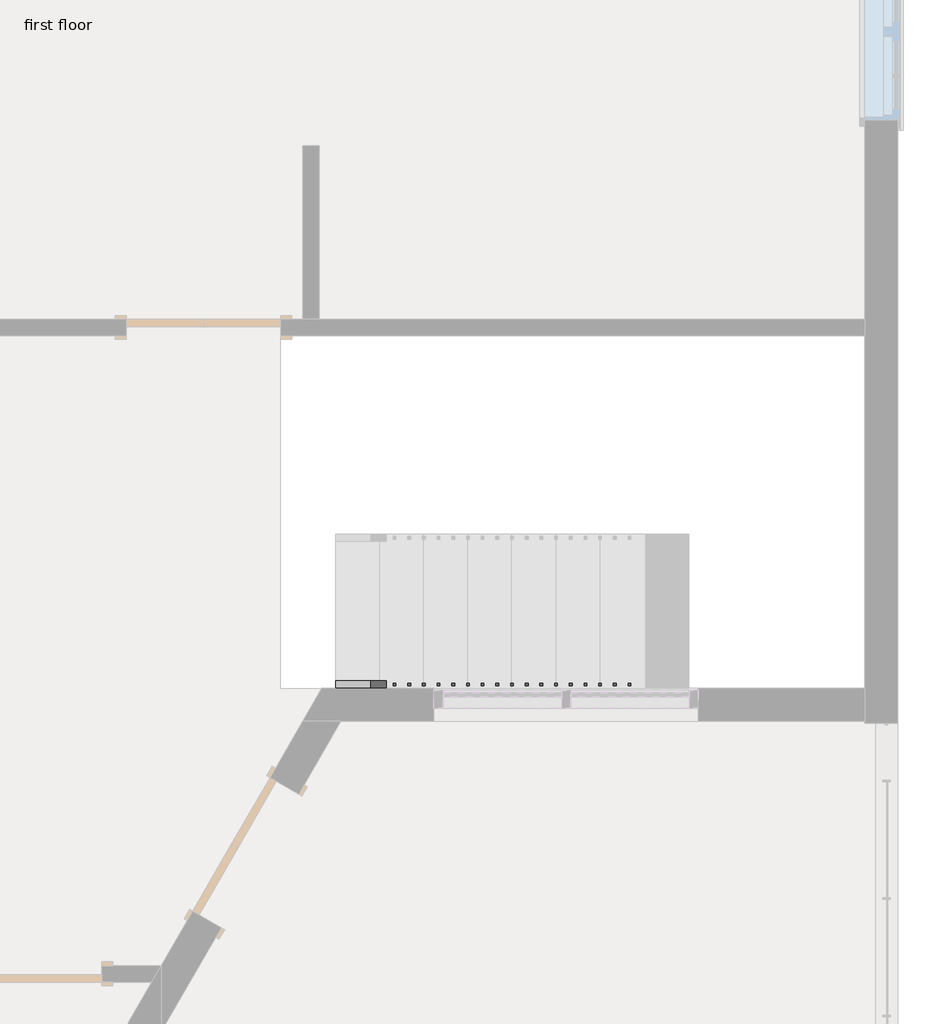
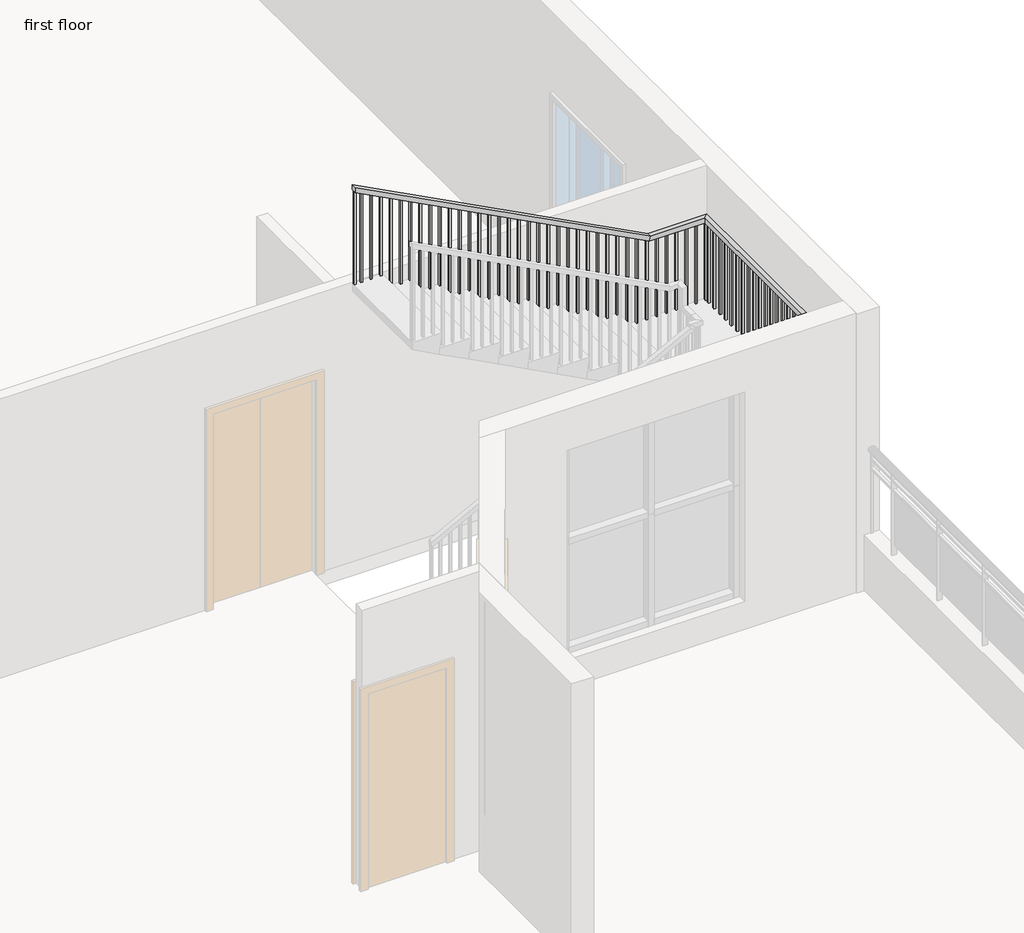
# One storey, part 3 of 4: 1 railing.
"""IFC4 building model written with IfcOpenShell, lengths in millimetres."""

from ifc_helpers import new_model, si_unit, frame, origin, place, context, project, spatial, polyline, outline, extrude, faceted_brep, element, save

model = new_model("IFC4")

# Units and contexts
model_context = context("Model", 3, world=origin())
ifc_project = project(units=[si_unit("LENGTHUNIT", "METRE", prefix="MILLI")], contexts=[model_context])

# Site, building, storey
site = spatial("IfcSite", under=ifc_project)
building = spatial("IfcBuilding", under=site)
storey = spatial("IfcBuildingStorey", under=building, Name="first floor", Elevation=3200.4)

# Railing
placement = place(None, origin())
element("IfcRailing", 1, ObjectType="Handrail - Rectangular", at=placement, inside=storey, context=model_context, shape_type="SolidModel", body=[
    faceted_brep([(1011.2585096, -3532.7523906, 4274.82), (1011.2585096, -3532.7523906, 4217.4446664), (1011.2585096, -3583.5523906, 4217.4446664), (1011.2585096, -3583.5523906, 4274.82), (3754.4585096, -3532.7523906, 5715.0), (3766.9829544, -3532.7523906, 5664.2), (3766.9829544, -3583.5523906, 5664.2), (3754.4585096, -3583.5523906, 5715.0), (4618.0585096, -3532.7523906, 5715.0), (4618.0585096, -3532.7523906, 5664.2), (4668.8585096, -3583.5523906, 5664.2), (4668.8585096, -3583.5523906, 5715.0), (4618.0585096, -1195.9523906, 5715.0), (4618.0585096, -1195.9523906, 5664.2), (4668.8585096, -1145.1523906, 5664.2), (4668.8585096, -1145.1523906, 5715.0), (4059.2585096, -1195.9523906, 5715.0), (4046.7340647, -1195.9523906, 5664.2), (4046.7340647, -1145.1523906, 5664.2), (4059.2585096, -1145.1523906, 5715.0), (1011.2585096, -1195.9523906, 7315.2), (1011.2585096, -1145.1523906, 7315.2), (1011.2585096, -1145.1523906, 7257.8246664), (1011.2585096, -1195.9523906, 7257.8246664)], [[[0, 1, 2, 3]], [[1, 0, 4, 5]], [[2, 1, 5, 6]], [[3, 2, 6, 7]], [[0, 3, 7, 4]], [[5, 4, 8, 9]], [[6, 5, 9, 10]], [[7, 6, 10, 11]], [[4, 7, 11, 8]], [[9, 8, 12, 13]], [[10, 9, 13, 14]], [[11, 10, 14, 15]], [[8, 11, 15, 12]], [[13, 12, 16, 17]], [[14, 13, 17, 18]], [[15, 14, 18, 19]], [[12, 15, 19, 16]], [[20, 21, 22, 23]], [[17, 16, 20, 23]], [[18, 17, 23, 22]], [[19, 18, 22, 21]], [[16, 19, 21, 20]]]),
    extrude(outline(polyline([(7212.8190414, 1096.9835096), (7222.8202914, 1077.9335096), (6240.78, 1077.9335096), (6240.78, 1096.9835096), (7212.8190414, 1096.9835096)])), frame((0.0, -1180.0773906, 0.0), z_axis=(0.0, 1.0, 0.0), x_axis=(0.0, 0.0, 1.0)), (0.0, 0.0, 1.0), 19.05),
    extrude(outline(polyline([(7159.4790414, 1198.5835096), (7169.4802914, 1179.5335096), (6240.78, 1179.5335096), (6240.78, 1198.5835096), (7159.4790414, 1198.5835096)])), frame((0.0, -1180.0773906, 0.0), z_axis=(0.0, 1.0, 0.0), x_axis=(0.0, 0.0, 1.0)), (0.0, 0.0, 1.0), 19.05),
    extrude(outline(polyline([(7106.1390414, 1300.1835096), (7116.1402914, 1281.1335096), (6240.78, 1281.1335096), (6240.78, 1300.1835096), (7106.1390414, 1300.1835096)])), frame((0.0, -1180.0773906, 0.0), z_axis=(0.0, 1.0, 0.0), x_axis=(0.0, 0.0, 1.0)), (0.0, 0.0, 1.0), 19.05),
    extrude(outline(polyline([(7052.7990414, 1401.7835096), (7062.8002914, 1382.7335096), (6080.76, 1382.7335096), (6080.76, 1401.7835096), (7052.7990414, 1401.7835096)])), frame((0.0, -1180.0773906, 0.0), z_axis=(0.0, 1.0, 0.0), x_axis=(0.0, 0.0, 1.0)), (0.0, 0.0, 1.0), 19.05),
    extrude(outline(polyline([(6999.4590414, 1503.3835096), (7009.4602914, 1484.3335096), (6080.76, 1484.3335096), (6080.76, 1503.3835096), (6999.4590414, 1503.3835096)])), frame((0.0, -1180.0773906, 0.0), z_axis=(0.0, 1.0, 0.0), x_axis=(0.0, 0.0, 1.0)), (0.0, 0.0, 1.0), 19.05),
    extrude(outline(polyline([(6946.1190414, 1604.9835096), (6956.1202914, 1585.9335096), (6080.76, 1585.9335096), (6080.76, 1604.9835096), (6946.1190414, 1604.9835096)])), frame((0.0, -1180.0773906, 0.0), z_axis=(0.0, 1.0, 0.0), x_axis=(0.0, 0.0, 1.0)), (0.0, 0.0, 1.0), 19.05),
    extrude(outline(polyline([(6892.7790414, 1706.5835096), (6902.7802914, 1687.5335096), (5920.74, 1687.5335096), (5920.74, 1706.5835096), (6892.7790414, 1706.5835096)])), frame((0.0, -1180.0773906, 0.0), z_axis=(0.0, 1.0, 0.0), x_axis=(0.0, 0.0, 1.0)), (0.0, 0.0, 1.0), 19.05),
    extrude(outline(polyline([(6839.4390414, 1808.1835096), (6849.4402914, 1789.1335096), (5920.74, 1789.1335096), (5920.74, 1808.1835096), (6839.4390414, 1808.1835096)])), frame((0.0, -1180.0773906, 0.0), z_axis=(0.0, 1.0, 0.0), x_axis=(0.0, 0.0, 1.0)), (0.0, 0.0, 1.0), 19.05),
    extrude(outline(polyline([(6786.0990414, 1909.7835096), (6796.1002914, 1890.7335096), (5920.74, 1890.7335096), (5920.74, 1909.7835096), (6786.0990414, 1909.7835096)])), frame((0.0, -1180.0773906, 0.0), z_axis=(0.0, 1.0, 0.0), x_axis=(0.0, 0.0, 1.0)), (0.0, 0.0, 1.0), 19.05),
    extrude(outline(polyline([(6732.7590414, 2011.3835096), (6742.7602914, 1992.3335096), (5760.72, 1992.3335096), (5760.72, 2011.3835096), (6732.7590414, 2011.3835096)])), frame((0.0, -1180.0773906, 0.0), z_axis=(0.0, 1.0, 0.0), x_axis=(0.0, 0.0, 1.0)), (0.0, 0.0, 1.0), 19.05),
    extrude(outline(polyline([(6679.4190414, 2112.9835096), (6689.4202914, 2093.9335096), (5760.72, 2093.9335096), (5760.72, 2112.9835096), (6679.4190414, 2112.9835096)])), frame((0.0, -1180.0773906, 0.0), z_axis=(0.0, 1.0, 0.0), x_axis=(0.0, 0.0, 1.0)), (0.0, 0.0, 1.0), 19.05),
    extrude(outline(polyline([(6626.0790414, 2214.5835096), (6636.0802914, 2195.5335096), (5760.72, 2195.5335096), (5760.72, 2214.5835096), (6626.0790414, 2214.5835096)])), frame((0.0, -1180.0773906, 0.0), z_axis=(0.0, 1.0, 0.0), x_axis=(0.0, 0.0, 1.0)), (0.0, 0.0, 1.0), 19.05),
    extrude(outline(polyline([(6572.7390414, 2316.1835096), (6582.7402914, 2297.1335096), (5600.7, 2297.1335096), (5600.7, 2316.1835096), (6572.7390414, 2316.1835096)])), frame((0.0, -1180.0773906, 0.0), z_axis=(0.0, 1.0, 0.0), x_axis=(0.0, 0.0, 1.0)), (0.0, 0.0, 1.0), 19.05),
    extrude(outline(polyline([(6519.3990414, 2417.7835096), (6529.4002914, 2398.7335096), (5600.7, 2398.7335096), (5600.7, 2417.7835096), (6519.3990414, 2417.7835096)])), frame((0.0, -1180.0773906, 0.0), z_axis=(0.0, 1.0, 0.0), x_axis=(0.0, 0.0, 1.0)), (0.0, 0.0, 1.0), 19.05),
    extrude(outline(polyline([(6466.0590414, 2519.3835096), (6476.0602914, 2500.3335096), (5600.7, 2500.3335096), (5600.7, 2519.3835096), (6466.0590414, 2519.3835096)])), frame((0.0, -1180.0773906, 0.0), z_axis=(0.0, 1.0, 0.0), x_axis=(0.0, 0.0, 1.0)), (0.0, 0.0, 1.0), 19.05),
    extrude(outline(polyline([(6412.7190414, 2620.9835096), (6422.7202914, 2601.9335096), (5440.68, 2601.9335096), (5440.68, 2620.9835096), (6412.7190414, 2620.9835096)])), frame((0.0, -1180.0773906, 0.0), z_axis=(0.0, 1.0, 0.0), x_axis=(0.0, 0.0, 1.0)), (0.0, 0.0, 1.0), 19.05),
    extrude(outline(polyline([(6359.3790414, 2722.5835096), (6369.3802914, 2703.5335096), (5440.68, 2703.5335096), (5440.68, 2722.5835096), (6359.3790414, 2722.5835096)])), frame((0.0, -1180.0773906, 0.0), z_axis=(0.0, 1.0, 0.0), x_axis=(0.0, 0.0, 1.0)), (0.0, 0.0, 1.0), 19.05),
    extrude(outline(polyline([(6306.0390414, 2824.1835096), (6316.0402914, 2805.1335096), (5440.68, 2805.1335096), (5440.68, 2824.1835096), (6306.0390414, 2824.1835096)])), frame((0.0, -1180.0773906, 0.0), z_axis=(0.0, 1.0, 0.0), x_axis=(0.0, 0.0, 1.0)), (0.0, 0.0, 1.0), 19.05),
    extrude(outline(polyline([(6252.6990414, 2925.7835096), (6262.7002914, 2906.7335096), (5280.66, 2906.7335096), (5280.66, 2925.7835096), (6252.6990414, 2925.7835096)])), frame((0.0, -1180.0773906, 0.0), z_axis=(0.0, 1.0, 0.0), x_axis=(0.0, 0.0, 1.0)), (0.0, 0.0, 1.0), 19.05),
    extrude(outline(polyline([(6199.3590414, 3027.3835096), (6209.3602914, 3008.3335096), (5280.66, 3008.3335096), (5280.66, 3027.3835096), (6199.3590414, 3027.3835096)])), frame((0.0, -1180.0773906, 0.0), z_axis=(0.0, 1.0, 0.0), x_axis=(0.0, 0.0, 1.0)), (0.0, 0.0, 1.0), 19.05),
    extrude(outline(polyline([(6146.0190414, 3128.9835096), (6156.0202914, 3109.9335096), (5280.66, 3109.9335096), (5280.66, 3128.9835096), (6146.0190414, 3128.9835096)])), frame((0.0, -1180.0773906, 0.0), z_axis=(0.0, 1.0, 0.0), x_axis=(0.0, 0.0, 1.0)), (0.0, 0.0, 1.0), 19.05),
    extrude(outline(polyline([(6092.6790414, 3230.5835096), (6102.6802914, 3211.5335096), (5120.64, 3211.5335096), (5120.64, 3230.5835096), (6092.6790414, 3230.5835096)])), frame((0.0, -1180.0773906, 0.0), z_axis=(0.0, 1.0, 0.0), x_axis=(0.0, 0.0, 1.0)), (0.0, 0.0, 1.0), 19.05),
    extrude(outline(polyline([(6039.3390414, 3332.1835096), (6049.3402914, 3313.1335096), (5120.64, 3313.1335096), (5120.64, 3332.1835096), (6039.3390414, 3332.1835096)])), frame((0.0, -1180.0773906, 0.0), z_axis=(0.0, 1.0, 0.0), x_axis=(0.0, 0.0, 1.0)), (0.0, 0.0, 1.0), 19.05),
    extrude(outline(polyline([(5985.9990414, 3433.7835096), (5996.0002914, 3414.7335096), (5120.64, 3414.7335096), (5120.64, 3433.7835096), (5985.9990414, 3433.7835096)])), frame((0.0, -1180.0773906, 0.0), z_axis=(0.0, 1.0, 0.0), x_axis=(0.0, 0.0, 1.0)), (0.0, 0.0, 1.0), 19.05),
    extrude(outline(polyline([(5932.6590414, 3535.3835096), (5942.6602914, 3516.3335096), (4960.62, 3516.3335096), (4960.62, 3535.3835096), (5932.6590414, 3535.3835096)])), frame((0.0, -1180.0773906, 0.0), z_axis=(0.0, 1.0, 0.0), x_axis=(0.0, 0.0, 1.0)), (0.0, 0.0, 1.0), 19.05),
    extrude(outline(polyline([(5879.3190414, 3636.9835096), (5889.3202914, 3617.9335096), (4960.62, 3617.9335096), (4960.62, 3636.9835096), (5879.3190414, 3636.9835096)])), frame((0.0, -1180.0773906, 0.0), z_axis=(0.0, 1.0, 0.0), x_axis=(0.0, 0.0, 1.0)), (0.0, 0.0, 1.0), 19.05),
    extrude(outline(polyline([(5825.9790414, 3738.5835096), (5835.9802914, 3719.5335096), (4960.62, 3719.5335096), (4960.62, 3738.5835096), (5825.9790414, 3738.5835096)])), frame((0.0, -1180.0773906, 0.0), z_axis=(0.0, 1.0, 0.0), x_axis=(0.0, 0.0, 1.0)), (0.0, 0.0, 1.0), 19.05),
    extrude(outline(polyline([(5772.6390414, 3840.1835096), (5782.6402914, 3821.1335096), (4800.6, 3821.1335096), (4800.6, 3840.1835096), (5772.6390414, 3840.1835096)])), frame((0.0, -1180.0773906, 0.0), z_axis=(0.0, 1.0, 0.0), x_axis=(0.0, 0.0, 1.0)), (0.0, 0.0, 1.0), 19.05),
    extrude(outline(polyline([(5719.2990414, 3941.7835096), (5729.3002914, 3922.7335096), (4800.6, 3922.7335096), (4800.6, 3941.7835096), (5719.2990414, 3941.7835096)])), frame((0.0, -1180.0773906, 0.0), z_axis=(0.0, 1.0, 0.0), x_axis=(0.0, 0.0, 1.0)), (0.0, 0.0, 1.0), 19.05),
    extrude(outline(polyline([(5665.9590414, 4043.3835096), (5675.9602914, 4024.3335096), (4800.6, 4024.3335096), (4800.6, 4043.3835096), (5665.9590414, 4043.3835096)])), frame((0.0, -1180.0773906, 0.0), z_axis=(0.0, 1.0, 0.0), x_axis=(0.0, 0.0, 1.0)), (0.0, 0.0, 1.0), 19.05),
    extrude(outline(polyline([(4144.9835096, -1161.0273906), (4144.9835096, -1180.0773906), (4125.9335096, -1180.0773906), (4125.9335096, -1161.0273906), (4144.9835096, -1161.0273906)])), frame((0.0, 0.0, 4800.6), z_axis=(0.0, 0.0, 1.0), x_axis=(1.0, 0.0, 0.0)), (0.0, 0.0, 1.0), 863.6),
    extrude(outline(polyline([(4246.5835096, -1161.0273906), (4246.5835096, -1180.0773906), (4227.5335096, -1180.0773906), (4227.5335096, -1161.0273906), (4246.5835096, -1161.0273906)])), frame((0.0, 0.0, 4800.6), z_axis=(0.0, 0.0, 1.0), x_axis=(1.0, 0.0, 0.0)), (0.0, 0.0, 1.0), 863.6),
    extrude(outline(polyline([(4348.1835096, -1161.0273906), (4348.1835096, -1180.0773906), (4329.1335096, -1180.0773906), (4329.1335096, -1161.0273906), (4348.1835096, -1161.0273906)])), frame((0.0, 0.0, 4800.6), z_axis=(0.0, 0.0, 1.0), x_axis=(1.0, 0.0, 0.0)), (0.0, 0.0, 1.0), 863.6),
    extrude(outline(polyline([(4449.7835096, -1161.0273906), (4449.7835096, -1180.0773906), (4430.7335096, -1180.0773906), (4430.7335096, -1161.0273906), (4449.7835096, -1161.0273906)])), frame((0.0, 0.0, 4800.6), z_axis=(0.0, 0.0, 1.0), x_axis=(1.0, 0.0, 0.0)), (0.0, 0.0, 1.0), 863.6),
    extrude(outline(polyline([(4551.3835096, -1161.0273906), (4551.3835096, -1180.0773906), (4532.3335096, -1180.0773906), (4532.3335096, -1161.0273906), (4551.3835096, -1161.0273906)])), frame((0.0, 0.0, 4800.6), z_axis=(0.0, 0.0, 1.0), x_axis=(1.0, 0.0, 0.0)), (0.0, 0.0, 1.0), 863.6),
    extrude(outline(polyline([(4652.9835096, -1230.8773906), (4633.9335096, -1230.8773906), (4633.9335096, -1211.8273906), (4652.9835096, -1211.8273906), (4652.9835096, -1230.8773906)])), frame((0.0, 0.0, 4800.6), z_axis=(0.0, 0.0, 1.0), x_axis=(1.0, 0.0, 0.0)), (0.0, 0.0, 1.0), 863.6),
    extrude(outline(polyline([(4652.9835096, -1332.4773906), (4633.9335096, -1332.4773906), (4633.9335096, -1313.4273906), (4652.9835096, -1313.4273906), (4652.9835096, -1332.4773906)])), frame((0.0, 0.0, 4800.6), z_axis=(0.0, 0.0, 1.0), x_axis=(1.0, 0.0, 0.0)), (0.0, 0.0, 1.0), 863.6),
    extrude(outline(polyline([(4652.9835096, -1434.0773906), (4633.9335096, -1434.0773906), (4633.9335096, -1415.0273906), (4652.9835096, -1415.0273906), (4652.9835096, -1434.0773906)])), frame((0.0, 0.0, 4800.6), z_axis=(0.0, 0.0, 1.0), x_axis=(1.0, 0.0, 0.0)), (0.0, 0.0, 1.0), 863.6),
    extrude(outline(polyline([(4652.9835096, -1535.6773906), (4633.9335096, -1535.6773906), (4633.9335096, -1516.6273906), (4652.9835096, -1516.6273906), (4652.9835096, -1535.6773906)])), frame((0.0, 0.0, 4800.6), z_axis=(0.0, 0.0, 1.0), x_axis=(1.0, 0.0, 0.0)), (0.0, 0.0, 1.0), 863.6),
    extrude(outline(polyline([(4652.9835096, -1637.2773906), (4633.9335096, -1637.2773906), (4633.9335096, -1618.2273906), (4652.9835096, -1618.2273906), (4652.9835096, -1637.2773906)])), frame((0.0, 0.0, 4800.6), z_axis=(0.0, 0.0, 1.0), x_axis=(1.0, 0.0, 0.0)), (0.0, 0.0, 1.0), 863.6),
    extrude(outline(polyline([(4652.9835096, -1738.8773906), (4633.9335096, -1738.8773906), (4633.9335096, -1719.8273906), (4652.9835096, -1719.8273906), (4652.9835096, -1738.8773906)])), frame((0.0, 0.0, 4800.6), z_axis=(0.0, 0.0, 1.0), x_axis=(1.0, 0.0, 0.0)), (0.0, 0.0, 1.0), 863.6),
    extrude(outline(polyline([(4652.9835096, -1840.4773906), (4633.9335096, -1840.4773906), (4633.9335096, -1821.4273906), (4652.9835096, -1821.4273906), (4652.9835096, -1840.4773906)])), frame((0.0, 0.0, 4800.6), z_axis=(0.0, 0.0, 1.0), x_axis=(1.0, 0.0, 0.0)), (0.0, 0.0, 1.0), 863.6),
    extrude(outline(polyline([(4652.9835096, -1942.0773906), (4633.9335096, -1942.0773906), (4633.9335096, -1923.0273906), (4652.9835096, -1923.0273906), (4652.9835096, -1942.0773906)])), frame((0.0, 0.0, 4800.6), z_axis=(0.0, 0.0, 1.0), x_axis=(1.0, 0.0, 0.0)), (0.0, 0.0, 1.0), 863.6),
    extrude(outline(polyline([(4652.9835096, -2043.6773906), (4633.9335096, -2043.6773906), (4633.9335096, -2024.6273906), (4652.9835096, -2024.6273906), (4652.9835096, -2043.6773906)])), frame((0.0, 0.0, 4800.6), z_axis=(0.0, 0.0, 1.0), x_axis=(1.0, 0.0, 0.0)), (0.0, 0.0, 1.0), 863.6),
    extrude(outline(polyline([(4652.9835096, -2145.2773906), (4633.9335096, -2145.2773906), (4633.9335096, -2126.2273906), (4652.9835096, -2126.2273906), (4652.9835096, -2145.2773906)])), frame((0.0, 0.0, 4800.6), z_axis=(0.0, 0.0, 1.0), x_axis=(1.0, 0.0, 0.0)), (0.0, 0.0, 1.0), 863.6),
    extrude(outline(polyline([(4652.9835096, -2246.8773906), (4633.9335096, -2246.8773906), (4633.9335096, -2227.8273906), (4652.9835096, -2227.8273906), (4652.9835096, -2246.8773906)])), frame((0.0, 0.0, 4800.6), z_axis=(0.0, 0.0, 1.0), x_axis=(1.0, 0.0, 0.0)), (0.0, 0.0, 1.0), 863.6),
    extrude(outline(polyline([(4652.9835096, -2348.4773906), (4633.9335096, -2348.4773906), (4633.9335096, -2329.4273906), (4652.9835096, -2329.4273906), (4652.9835096, -2348.4773906)])), frame((0.0, 0.0, 4800.6), z_axis=(0.0, 0.0, 1.0), x_axis=(1.0, 0.0, 0.0)), (0.0, 0.0, 1.0), 863.6),
    extrude(outline(polyline([(4652.9835096, -2450.0773906), (4633.9335096, -2450.0773906), (4633.9335096, -2431.0273906), (4652.9835096, -2431.0273906), (4652.9835096, -2450.0773906)])), frame((0.0, 0.0, 4800.6), z_axis=(0.0, 0.0, 1.0), x_axis=(1.0, 0.0, 0.0)), (0.0, 0.0, 1.0), 863.6),
    extrude(outline(polyline([(4652.9835096, -2551.6773906), (4633.9335096, -2551.6773906), (4633.9335096, -2532.6273906), (4652.9835096, -2532.6273906), (4652.9835096, -2551.6773906)])), frame((0.0, 0.0, 4800.6), z_axis=(0.0, 0.0, 1.0), x_axis=(1.0, 0.0, 0.0)), (0.0, 0.0, 1.0), 863.6),
    extrude(outline(polyline([(4652.9835096, -2653.2773906), (4633.9335096, -2653.2773906), (4633.9335096, -2634.2273906), (4652.9835096, -2634.2273906), (4652.9835096, -2653.2773906)])), frame((0.0, 0.0, 4800.6), z_axis=(0.0, 0.0, 1.0), x_axis=(1.0, 0.0, 0.0)), (0.0, 0.0, 1.0), 863.6),
    extrude(outline(polyline([(4652.9835096, -2754.8773906), (4633.9335096, -2754.8773906), (4633.9335096, -2735.8273906), (4652.9835096, -2735.8273906), (4652.9835096, -2754.8773906)])), frame((0.0, 0.0, 4800.6), z_axis=(0.0, 0.0, 1.0), x_axis=(1.0, 0.0, 0.0)), (0.0, 0.0, 1.0), 863.6),
    extrude(outline(polyline([(4652.9835096, -2856.4773906), (4633.9335096, -2856.4773906), (4633.9335096, -2837.4273906), (4652.9835096, -2837.4273906), (4652.9835096, -2856.4773906)])), frame((0.0, 0.0, 4800.6), z_axis=(0.0, 0.0, 1.0), x_axis=(1.0, 0.0, 0.0)), (0.0, 0.0, 1.0), 863.6),
    extrude(outline(polyline([(4652.9835096, -2958.0773906), (4633.9335096, -2958.0773906), (4633.9335096, -2939.0273906), (4652.9835096, -2939.0273906), (4652.9835096, -2958.0773906)])), frame((0.0, 0.0, 4800.6), z_axis=(0.0, 0.0, 1.0), x_axis=(1.0, 0.0, 0.0)), (0.0, 0.0, 1.0), 863.6),
    extrude(outline(polyline([(4652.9835096, -3059.6773906), (4633.9335096, -3059.6773906), (4633.9335096, -3040.6273906), (4652.9835096, -3040.6273906), (4652.9835096, -3059.6773906)])), frame((0.0, 0.0, 4800.6), z_axis=(0.0, 0.0, 1.0), x_axis=(1.0, 0.0, 0.0)), (0.0, 0.0, 1.0), 863.6),
    extrude(outline(polyline([(4652.9835096, -3161.2773906), (4633.9335096, -3161.2773906), (4633.9335096, -3142.2273906), (4652.9835096, -3142.2273906), (4652.9835096, -3161.2773906)])), frame((0.0, 0.0, 4800.6), z_axis=(0.0, 0.0, 1.0), x_axis=(1.0, 0.0, 0.0)), (0.0, 0.0, 1.0), 863.6),
    extrude(outline(polyline([(4652.9835096, -3262.8773906), (4633.9335096, -3262.8773906), (4633.9335096, -3243.8273906), (4652.9835096, -3243.8273906), (4652.9835096, -3262.8773906)])), frame((0.0, 0.0, 4800.6), z_axis=(0.0, 0.0, 1.0), x_axis=(1.0, 0.0, 0.0)), (0.0, 0.0, 1.0), 863.6),
    extrude(outline(polyline([(4652.9835096, -3364.4773906), (4633.9335096, -3364.4773906), (4633.9335096, -3345.4273906), (4652.9835096, -3345.4273906), (4652.9835096, -3364.4773906)])), frame((0.0, 0.0, 4800.6), z_axis=(0.0, 0.0, 1.0), x_axis=(1.0, 0.0, 0.0)), (0.0, 0.0, 1.0), 863.6),
    extrude(outline(polyline([(4652.9835096, -3466.0773906), (4633.9335096, -3466.0773906), (4633.9335096, -3447.0273906), (4652.9835096, -3447.0273906), (4652.9835096, -3466.0773906)])), frame((0.0, 0.0, 4800.6), z_axis=(0.0, 0.0, 1.0), x_axis=(1.0, 0.0, 0.0)), (0.0, 0.0, 1.0), 863.6),
    extrude(outline(polyline([(4557.7335096, -3567.6773906), (4557.7335096, -3548.6273906), (4576.7835096, -3548.6273906), (4576.7835096, -3567.6773906), (4557.7335096, -3567.6773906)])), frame((0.0, 0.0, 4800.6), z_axis=(0.0, 0.0, 1.0), x_axis=(1.0, 0.0, 0.0)), (0.0, 0.0, 1.0), 863.6),
    extrude(outline(polyline([(4456.1335096, -3567.6773906), (4456.1335096, -3548.6273906), (4475.1835096, -3548.6273906), (4475.1835096, -3567.6773906), (4456.1335096, -3567.6773906)])), frame((0.0, 0.0, 4800.6), z_axis=(0.0, 0.0, 1.0), x_axis=(1.0, 0.0, 0.0)), (0.0, 0.0, 1.0), 863.6),
    extrude(outline(polyline([(4354.5335096, -3567.6773906), (4354.5335096, -3548.6273906), (4373.5835096, -3548.6273906), (4373.5835096, -3567.6773906), (4354.5335096, -3567.6773906)])), frame((0.0, 0.0, 4800.6), z_axis=(0.0, 0.0, 1.0), x_axis=(1.0, 0.0, 0.0)), (0.0, 0.0, 1.0), 863.6),
    extrude(outline(polyline([(4252.9335096, -3567.6773906), (4252.9335096, -3548.6273906), (4271.9835096, -3548.6273906), (4271.9835096, -3567.6773906), (4252.9335096, -3567.6773906)])), frame((0.0, 0.0, 4800.6), z_axis=(0.0, 0.0, 1.0), x_axis=(1.0, 0.0, 0.0)), (0.0, 0.0, 1.0), 863.6),
    extrude(outline(polyline([(4151.3335096, -3567.6773906), (4151.3335096, -3548.6273906), (4170.3835096, -3548.6273906), (4170.3835096, -3567.6773906), (4151.3335096, -3567.6773906)])), frame((0.0, 0.0, 4800.6), z_axis=(0.0, 0.0, 1.0), x_axis=(1.0, 0.0, 0.0)), (0.0, 0.0, 1.0), 863.6),
    extrude(outline(polyline([(4049.7335096, -3567.6773906), (4049.7335096, -3548.6273906), (4068.7835096, -3548.6273906), (4068.7835096, -3567.6773906), (4049.7335096, -3567.6773906)])), frame((0.0, 0.0, 4800.6), z_axis=(0.0, 0.0, 1.0), x_axis=(1.0, 0.0, 0.0)), (0.0, 0.0, 1.0), 863.6),
    extrude(outline(polyline([(3948.1335096, -3567.6773906), (3948.1335096, -3548.6273906), (3967.1835096, -3548.6273906), (3967.1835096, -3567.6773906), (3948.1335096, -3567.6773906)])), frame((0.0, 0.0, 4800.6), z_axis=(0.0, 0.0, 1.0), x_axis=(1.0, 0.0, 0.0)), (0.0, 0.0, 1.0), 863.6),
    extrude(outline(polyline([(3846.5335096, -3567.6773906), (3846.5335096, -3548.6273906), (3865.5835096, -3548.6273906), (3865.5835096, -3567.6773906), (3846.5335096, -3567.6773906)])), frame((0.0, 0.0, 4800.6), z_axis=(0.0, 0.0, 1.0), x_axis=(1.0, 0.0, 0.0)), (0.0, 0.0, 1.0), 863.6),
    extrude(outline(polyline([(5662.6252914, 3763.9835096), (5652.6240414, 3744.9335096), (4800.6, 3744.9335096), (4800.6, 3763.9835096), (5662.6252914, 3763.9835096)])), frame((0.0, -3567.6773906, 0.0), z_axis=(0.0, 1.0, 0.0), x_axis=(0.0, 0.0, 1.0)), (0.0, 0.0, 1.0), 19.05),
    extrude(outline(polyline([(5609.2852914, 3662.3835096), (5599.2840414, 3643.3335096), (4640.58, 3643.3335096), (4640.58, 3662.3835096), (5609.2852914, 3662.3835096)])), frame((0.0, -3567.6773906, 0.0), z_axis=(0.0, 1.0, 0.0), x_axis=(0.0, 0.0, 1.0)), (0.0, 0.0, 1.0), 19.05),
    extrude(outline(polyline([(5555.9452914, 3560.7835096), (5545.9440414, 3541.7335096), (4640.58, 3541.7335096), (4640.58, 3560.7835096), (5555.9452914, 3560.7835096)])), frame((0.0, -3567.6773906, 0.0), z_axis=(0.0, 1.0, 0.0), x_axis=(0.0, 0.0, 1.0)), (0.0, 0.0, 1.0), 19.05),
    extrude(outline(polyline([(5502.6052914, 3459.1835096), (5492.6040414, 3440.1335096), (4640.58, 3440.1335096), (4640.58, 3459.1835096), (5502.6052914, 3459.1835096)])), frame((0.0, -3567.6773906, 0.0), z_axis=(0.0, 1.0, 0.0), x_axis=(0.0, 0.0, 1.0)), (0.0, 0.0, 1.0), 19.05),
    extrude(outline(polyline([(5449.2652914, 3357.5835096), (5439.2640414, 3338.5335096), (4480.56, 3338.5335096), (4480.56, 3357.5835096), (5449.2652914, 3357.5835096)])), frame((0.0, -3567.6773906, 0.0), z_axis=(0.0, 1.0, 0.0), x_axis=(0.0, 0.0, 1.0)), (0.0, 0.0, 1.0), 19.05),
    extrude(outline(polyline([(5395.9252914, 3255.9835096), (5385.9240414, 3236.9335096), (4480.56, 3236.9335096), (4480.56, 3255.9835096), (5395.9252914, 3255.9835096)])), frame((0.0, -3567.6773906, 0.0), z_axis=(0.0, 1.0, 0.0), x_axis=(0.0, 0.0, 1.0)), (0.0, 0.0, 1.0), 19.05),
    extrude(outline(polyline([(5342.5852914, 3154.3835096), (5332.5840414, 3135.3335096), (4480.56, 3135.3335096), (4480.56, 3154.3835096), (5342.5852914, 3154.3835096)])), frame((0.0, -3567.6773906, 0.0), z_axis=(0.0, 1.0, 0.0), x_axis=(0.0, 0.0, 1.0)), (0.0, 0.0, 1.0), 19.05),
    extrude(outline(polyline([(5289.2452914, 3052.7835096), (5279.2440414, 3033.7335096), (4320.54, 3033.7335096), (4320.54, 3052.7835096), (5289.2452914, 3052.7835096)])), frame((0.0, -3567.6773906, 0.0), z_axis=(0.0, 1.0, 0.0), x_axis=(0.0, 0.0, 1.0)), (0.0, 0.0, 1.0), 19.05),
    extrude(outline(polyline([(5235.9052914, 2951.1835096), (5225.9040414, 2932.1335096), (4320.54, 2932.1335096), (4320.54, 2951.1835096), (5235.9052914, 2951.1835096)])), frame((0.0, -3567.6773906, 0.0), z_axis=(0.0, 1.0, 0.0), x_axis=(0.0, 0.0, 1.0)), (0.0, 0.0, 1.0), 19.05),
    extrude(outline(polyline([(5182.5652914, 2849.5835096), (5172.5640414, 2830.5335096), (4320.54, 2830.5335096), (4320.54, 2849.5835096), (5182.5652914, 2849.5835096)])), frame((0.0, -3567.6773906, 0.0), z_axis=(0.0, 1.0, 0.0), x_axis=(0.0, 0.0, 1.0)), (0.0, 0.0, 1.0), 19.05),
    extrude(outline(polyline([(5129.2252914, 2747.9835096), (5119.2240414, 2728.9335096), (4160.52, 2728.9335096), (4160.52, 2747.9835096), (5129.2252914, 2747.9835096)])), frame((0.0, -3567.6773906, 0.0), z_axis=(0.0, 1.0, 0.0), x_axis=(0.0, 0.0, 1.0)), (0.0, 0.0, 1.0), 19.05),
    extrude(outline(polyline([(5075.8852914, 2646.3835096), (5065.8840414, 2627.3335096), (4160.52, 2627.3335096), (4160.52, 2646.3835096), (5075.8852914, 2646.3835096)])), frame((0.0, -3567.6773906, 0.0), z_axis=(0.0, 1.0, 0.0), x_axis=(0.0, 0.0, 1.0)), (0.0, 0.0, 1.0), 19.05),
    extrude(outline(polyline([(5022.5452914, 2544.7835096), (5012.5440414, 2525.7335096), (4160.52, 2525.7335096), (4160.52, 2544.7835096), (5022.5452914, 2544.7835096)])), frame((0.0, -3567.6773906, 0.0), z_axis=(0.0, 1.0, 0.0), x_axis=(0.0, 0.0, 1.0)), (0.0, 0.0, 1.0), 19.05),
    extrude(outline(polyline([(4969.2052914, 2443.1835096), (4959.2040414, 2424.1335096), (4000.5, 2424.1335096), (4000.5, 2443.1835096), (4969.2052914, 2443.1835096)])), frame((0.0, -3567.6773906, 0.0), z_axis=(0.0, 1.0, 0.0), x_axis=(0.0, 0.0, 1.0)), (0.0, 0.0, 1.0), 19.05),
    extrude(outline(polyline([(4915.8652914, 2341.5835096), (4905.8640414, 2322.5335096), (4000.5, 2322.5335096), (4000.5, 2341.5835096), (4915.8652914, 2341.5835096)])), frame((0.0, -3567.6773906, 0.0), z_axis=(0.0, 1.0, 0.0), x_axis=(0.0, 0.0, 1.0)), (0.0, 0.0, 1.0), 19.05),
    extrude(outline(polyline([(4862.5252914, 2239.9835096), (4852.5240414, 2220.9335096), (4000.5, 2220.9335096), (4000.5, 2239.9835096), (4862.5252914, 2239.9835096)])), frame((0.0, -3567.6773906, 0.0), z_axis=(0.0, 1.0, 0.0), x_axis=(0.0, 0.0, 1.0)), (0.0, 0.0, 1.0), 19.05),
    extrude(outline(polyline([(4809.1852914, 2138.3835096), (4799.1840414, 2119.3335096), (3840.48, 2119.3335096), (3840.48, 2138.3835096), (4809.1852914, 2138.3835096)])), frame((0.0, -3567.6773906, 0.0), z_axis=(0.0, 1.0, 0.0), x_axis=(0.0, 0.0, 1.0)), (0.0, 0.0, 1.0), 19.05),
    extrude(outline(polyline([(4755.8452914, 2036.7835096), (4745.8440414, 2017.7335096), (3840.48, 2017.7335096), (3840.48, 2036.7835096), (4755.8452914, 2036.7835096)])), frame((0.0, -3567.6773906, 0.0), z_axis=(0.0, 1.0, 0.0), x_axis=(0.0, 0.0, 1.0)), (0.0, 0.0, 1.0), 19.05),
    extrude(outline(polyline([(4702.5052914, 1935.1835096), (4692.5040414, 1916.1335096), (3840.48, 1916.1335096), (3840.48, 1935.1835096), (4702.5052914, 1935.1835096)])), frame((0.0, -3567.6773906, 0.0), z_axis=(0.0, 1.0, 0.0), x_axis=(0.0, 0.0, 1.0)), (0.0, 0.0, 1.0), 19.05),
    extrude(outline(polyline([(4649.1652914, 1833.5835096), (4639.1640414, 1814.5335096), (3680.46, 1814.5335096), (3680.46, 1833.5835096), (4649.1652914, 1833.5835096)])), frame((0.0, -3567.6773906, 0.0), z_axis=(0.0, 1.0, 0.0), x_axis=(0.0, 0.0, 1.0)), (0.0, 0.0, 1.0), 19.05),
    extrude(outline(polyline([(4595.8252914, 1731.9835096), (4585.8240414, 1712.9335096), (3680.46, 1712.9335096), (3680.46, 1731.9835096), (4595.8252914, 1731.9835096)])), frame((0.0, -3567.6773906, 0.0), z_axis=(0.0, 1.0, 0.0), x_axis=(0.0, 0.0, 1.0)), (0.0, 0.0, 1.0), 19.05),
    extrude(outline(polyline([(4542.4852914, 1630.3835096), (4532.4840414, 1611.3335096), (3680.46, 1611.3335096), (3680.46, 1630.3835096), (4542.4852914, 1630.3835096)])), frame((0.0, -3567.6773906, 0.0), z_axis=(0.0, 1.0, 0.0), x_axis=(0.0, 0.0, 1.0)), (0.0, 0.0, 1.0), 19.05),
    extrude(outline(polyline([(4489.1452914, 1528.7835096), (4479.1440414, 1509.7335096), (3520.44, 1509.7335096), (3520.44, 1528.7835096), (4489.1452914, 1528.7835096)])), frame((0.0, -3567.6773906, 0.0), z_axis=(0.0, 1.0, 0.0), x_axis=(0.0, 0.0, 1.0)), (0.0, 0.0, 1.0), 19.05),
    extrude(outline(polyline([(4435.8052914, 1427.1835096), (4425.8040414, 1408.1335096), (3520.44, 1408.1335096), (3520.44, 1427.1835096), (4435.8052914, 1427.1835096)])), frame((0.0, -3567.6773906, 0.0), z_axis=(0.0, 1.0, 0.0), x_axis=(0.0, 0.0, 1.0)), (0.0, 0.0, 1.0), 19.05),
    extrude(outline(polyline([(4382.4652914, 1325.5835096), (4372.4640414, 1306.5335096), (3520.44, 1306.5335096), (3520.44, 1325.5835096), (4382.4652914, 1325.5835096)])), frame((0.0, -3567.6773906, 0.0), z_axis=(0.0, 1.0, 0.0), x_axis=(0.0, 0.0, 1.0)), (0.0, 0.0, 1.0), 19.05),
    extrude(outline(polyline([(4329.1252914, 1223.9835096), (4319.1240414, 1204.9335096), (3360.42, 1204.9335096), (3360.42, 1223.9835096), (4329.1252914, 1223.9835096)])), frame((0.0, -3567.6773906, 0.0), z_axis=(0.0, 1.0, 0.0), x_axis=(0.0, 0.0, 1.0)), (0.0, 0.0, 1.0), 19.05),
    extrude(outline(polyline([(4275.7852914, 1122.3835096), (4265.7840414, 1103.3335096), (3360.42, 1103.3335096), (3360.42, 1122.3835096), (4275.7852914, 1122.3835096)])), frame((0.0, -3567.6773906, 0.0), z_axis=(0.0, 1.0, 0.0), x_axis=(0.0, 0.0, 1.0)), (0.0, 0.0, 1.0), 19.05),
    extrude(outline(polyline([(4652.9835096, -1180.0773906), (4633.9335096, -1180.0773906), (4633.9335096, -1161.0273906), (4652.9835096, -1161.0273906), (4652.9835096, -1180.0773906)])), frame((0.0, 0.0, 4800.6), z_axis=(0.0, 0.0, 1.0), x_axis=(1.0, 0.0, 0.0)), (0.0, 0.0, 1.0), 863.6),
    extrude(outline(polyline([(4633.9335096, -3567.6773906), (4633.9335096, -3548.6273906), (4652.9835096, -3548.6273906), (4652.9835096, -3567.6773906), (4633.9335096, -3567.6773906)])), frame((0.0, 0.0, 4800.6), z_axis=(0.0, 0.0, 1.0), x_axis=(1.0, 0.0, 0.0)), (0.0, 0.0, 1.0), 863.6),
    extrude(outline(polyline([(7247.8234164, 1030.3085096), (7257.8246664, 1011.2585096), (6240.78, 1011.2585096), (6240.78, 1030.3085096), (7247.8234164, 1030.3085096)])), frame((0.0, -1180.0773906, 0.0), z_axis=(0.0, 1.0, 0.0), x_axis=(0.0, 0.0, 1.0)), (0.0, 0.0, 1.0), 19.05),
    extrude(outline(polyline([(4227.4459164, 1030.3085096), (4217.4446664, 1011.2585096), (3360.42, 1011.2585096), (3360.42, 1030.3085096), (4227.4459164, 1030.3085096)])), frame((0.0, -3567.6773906, 0.0), z_axis=(0.0, 1.0, 0.0), x_axis=(0.0, 0.0, 1.0)), (0.0, 0.0, 1.0), 19.05),
])

save(model, "model.ifc")

# Revit data of these elements
# Type "Handrail - Rectangular"
#   Assembly Code = "C2010400"
#   built-in parameter 1008612 = 0.0416667 (stored number, unit not read)
#   built-in parameter 1008611 = 0.0416667 (stored number, unit not read)
#   built-in parameter 1008609 = 0.333333 (stored number, unit not read)
#   built-in parameter 1008604 = 0.166667 (stored number, unit not read)
#   built-in parameter 1008603 = 0.166667 (stored number, unit not read)
#   Railing Height = 3' - 0"
#   built-in parameter 1008630 = 2
#   built-in parameter 1008610 = 2
#   built-in parameter 1008618 = Baluster - Square : 3/4"
# Element 1 (IfcRailing, "Handrail - Rectangular")
#   Phase Created = New Construction
